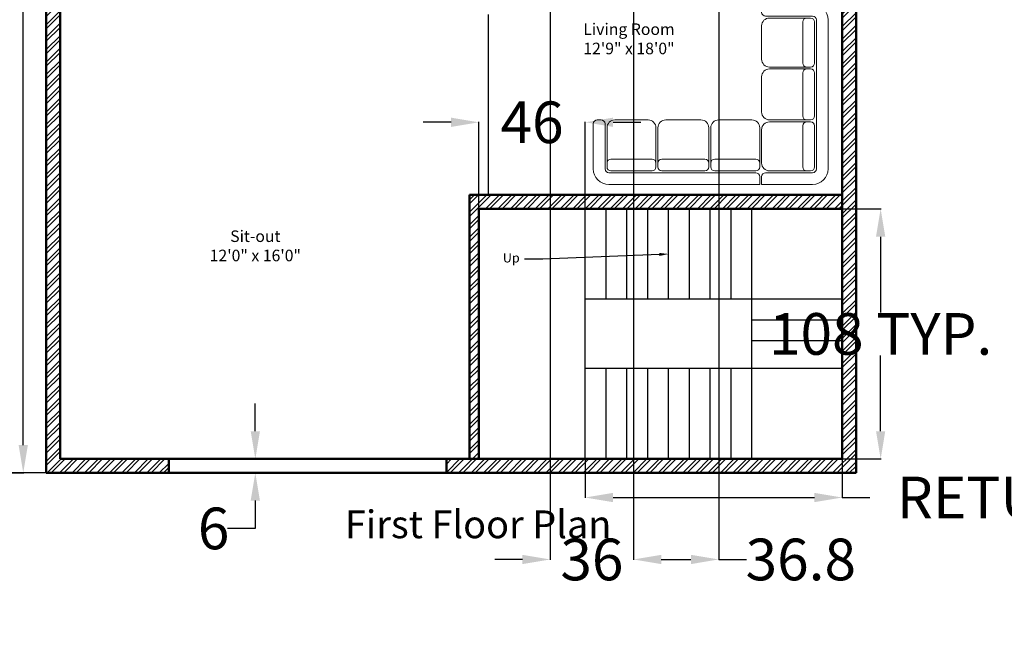
# Model space of a CAD drawing. Units: inches. Extents: x 73 to 1216, y -495 to 328.
# Tile 4 of 9: x 569 to 994, y -495 to -232. Entities that reach past the tile are written whole.
import ezdxf
from ezdxf import colors
from ezdxf.entities.mleader import LeaderData, LeaderLine
from ezdxf.math import Vec2, Vec3

# ---------------------------------------------------------------- set-up
doc = ezdxf.new("R2010")
doc.units = ezdxf.units.IN
for name, color, linetype, lineweight in [('A-ANNO-DIMS', 2, 'Continuous', 18), ('A-ANNO-TITL', 7, 'Continuous', 35), ('A-AREA-IDEN', 7, 'Continuous', 18), ('A-FLOR-EDGE', 7, 'Continuous', 25), ('A-WALL-PATT', 8, 'Continuous', 13), ('Furniture', 2, 'Continuous', 18), ('Outer Walls', 1, 'Continuous', 50), ('Stairs', 8, 'Continuous', 25), ('Text-T18', 7, 'Continuous', 18)]:
    doc.layers.add(name, color=color, linetype=linetype, lineweight=lineweight)
doc.styles.get("Standard").update_dxf_attribs({"font": 'arial.ttf'})
doc.dimstyles.get("Standard").update_dxf_attribs({"dimtxt": 18, "dimasz": 12, "dimexe": 0.18, "dimexo": 0.0625, "dimgap": 0.09, "dimtad": 0, "dimtih": 1, "dimtoh": 1, "dimdec": 0, "dimzin": 0, "dimdsep": 46, "dimlunit": 3, "dimtxsty": 'Standard', "dimcen": 0.09, "dimadec": 0, "dimazin": 0, "dimtfac": 1, "dimtdec": 0, "dimtofl": 0, "dimtmove": 0, "dimatfit": 3, "dimfxl": 1, "dimtolj": 1, "dimtzin": 0, "dimarcsym": 0})
pattern_1 = [(45, (-647.324, -1257.0093), (-2.694077, 2.694077), []), (45, (-645.528, -1257.0093), (-2.694077, 2.694077), [])]

# ---------------------------------------------------------------- blocks, each defined once
blk = doc.blocks.new('A$C2AFA021D')
for p, q in [((0.8, 2.3), (0.2, 2.3)), ((0.2, 2.15), (0.8, 2.15)), ((0.85, 2.2), (0.85, 2.25)), ((0, 2.1), (0, 0.2)), ((0.15, 0.2), (0.15, 2.1)), ((0.175, 1.55), (0.175, 2.075)), ((0.225, 2.125), (0.275, 2.125)), ((0.75, 2.125), (0.275, 2.125)), ((0.325, 2.075), (0.325, 1.55)), ((0.85, 1.6), (0.85, 2.025)), ((0.175, 0.875), (0.175, 1.425)), ((0.275, 1.5), (0.225, 1.5)), ((0.225, 1.475), (0.275, 1.475)), ((0.275, 1.5), (0.75, 1.5)), ((0.75, 1.475), (0.275, 1.475)), ((0.325, 1.425), (0.325, 0.875)), ((0.85, 0.925), (0.85, 1.375)), ((0.275, 0.825), (0.225, 0.825)), ((0.225, 0.8), (0.275, 0.8)), ((0.275, 0.825), (0.75, 0.825)), ((0.75, 0.8), (0.275, 0.8)), ((0.975, 0.825), (1.4, 0.825)), ((1.625, 0.825), (2.075, 0.825)), ((2.3, 0.825), (2.725, 0.825)), ((2.85, 0.2), (2.85, 0.775)), ((2.9, 0.825), (2.95, 0.825)), ((3, 0.775), (3, 0.2)), ((0.175, 0.225), (0.175, 0.75)), ((0.325, 0.75), (0.325, 0.225)), ((0.85, 0.275), (0.85, 0.7)), ((0.875, 0.275), (0.875, 0.725)), ((1.5, 0.725), (1.5, 0.275)), ((1.525, 0.275), (1.525, 0.725)), ((2.175, 0.725), (2.175, 0.275)), ((2.2, 0.275), (2.2, 0.725)), ((2.825, 0.725), (2.825, 0.275)), ((0.875, 0.275), (0.875, 0.225)), ((1.45, 0.325), (0.925, 0.325)), ((1.5, 0.225), (1.5, 0.275)), ((1.525, 0.275), (1.525, 0.225)), ((2.125, 0.325), (1.575, 0.325)), ((2.175, 0.225), (2.175, 0.275)), ((2.2, 0.275), (2.2, 0.225)), ((2.775, 0.325), (2.25, 0.325)), ((2.825, 0.225), (2.825, 0.275)), ((0.8, 0.15), (0.2, 0.15)), ((0.275, 0.175), (0.225, 0.175)), ((0.275, 0.175), (0.75, 0.175)), ((0.925, 0.175), (1.45, 0.175)), ((0.925, 0.15), (2.8, 0.15)), ((1.575, 0.175), (2.125, 0.175)), ((2.25, 0.175), (2.775, 0.175)), ((0.85, 0), (0.85, 0.1)), ((0.875, 0.1), (0.875, 0)), ((0.2, 0), (0.85, 0)), ((2.8, 0), (0.875, 0))]:
    blk.add_line(p, q)
for centre, radius, start, end in [((0.2, 2.1), 0.2, 90, 180), ((0.8, 2.25), 0.05, 0, 90), ((0.2, 2.1), 0.05, 90, 180), ((0.8, 2.2), 0.05, 270, 0), ((0.225, 2.075), 0.05, 90, 180), ((0.275, 2.075), 0.05, 0, 90), ((0.75, 2.025), 0.1, 0, 90), ((0.225, 1.55), 0.05, 180, 270), ((0.275, 1.55), 0.05, 270, 0), ((0.75, 1.6), 0.1, 270, 0), ((0.225, 1.425), 0.05, 90, 180), ((0.275, 1.425), 0.05, 0, 90), ((0.75, 1.375), 0.1, 360, 90), ((0.75, 0.925), 0.1, 270, 0), ((0.225, 0.875), 0.05, 180, 270), ((0.225, 0.75), 0.05, 90, 180), ((0.275, 0.875), 0.05, 270, 0), ((0.275, 0.75), 0.05, 0, 90), ((0.75, 0.7), 0.1, 0, 90), ((0.975, 0.725), 0.1, 90, 180), ((1.4, 0.725), 0.1, 0, 90), ((1.625, 0.725), 0.1, 90, 180), ((2.075, 0.725), 0.1, 0, 90), ((2.3, 0.725), 0.1, 90, 180), ((2.725, 0.725), 0.1, 0, 90), ((2.9, 0.775), 0.05, 90, 180), ((2.95, 0.775), 0.05, 0, 90), ((0.75, 0.275), 0.1, 270, 0), ((0.925, 0.275), 0.05, 90, 180), ((1.45, 0.275), 0.05, 360, 90), ((1.575, 0.275), 0.05, 90, 180), ((2.125, 0.275), 0.05, 360, 90), ((2.25, 0.275), 0.05, 90, 180), ((2.775, 0.275), 0.05, 360, 90), ((0.2, 0.2), 0.2, 180, 270), ((0.2, 0.2), 0.05, 180, 270), ((0.225, 0.225), 0.05, 180, 270), ((0.275, 0.225), 0.05, 270, 0), ((0.8, 0.1), 0.05, 0, 90), ((0.925, 0.225), 0.05, 180, 270), ((0.925, 0.1), 0.05, 90, 180), ((1.45, 0.225), 0.05, 270, 0), ((1.575, 0.225), 0.05, 180, 270), ((2.125, 0.225), 0.05, 270, 0), ((2.25, 0.225), 0.05, 180, 270), ((2.775, 0.225), 0.05, 270, 0), ((2.8, 0.2), 0.2, 270, 0), ((2.8, 0.2), 0.05, 270, 0)]:
    blk.add_arc(centre, radius, start, end)
blk = doc.blocks.new('STAIR-RETURN')
for p, q in [((0, 69), (0, 108)), ((9, 69), (9, 108)), ((18, 69), (18, 108)), ((27, 69), (27, 108)), ((36, 69), (36, 108)), ((45, 69), (45, 108)), ((54, 69), (54, 108)), ((63, 69), (63, 108)), ((72, 0), (72, 108)), ((111, 69), (0, 69)), ((0, 0), (0, 69)), ((111, 60), (72, 60)), ((111, 51), (72, 51)), ((111, 39), (0, 39)), ((9, 0), (9, 39)), ((18, 0), (18, 39)), ((27, 0), (27, 39)), ((36, 0), (36, 39)), ((45, 0), (45, 39)), ((54, 0), (54, 39)), ((63, 0), (63, 39))]:
    blk.add_line(p, q)
blk = doc.blocks.new('*D46')
at = {"layer": 'A-ANNO-DIMS', "color": 0, "lineweight": -2, "transparency": 16777216}
for p, q in [((813.16, -421.89), (813.16, -438.65)), ((924.16, -421.89), (924.16, -438.65)), ((825.16, -438.47), (912.16, -438.47)), ((924.16, -438.47), (936.16, -438.47))]:
    blk.add_line(p, q, dxfattribs=at)
at = {"layer": 'A-ANNO-DIMS', "color": 0, "transparency": 16777216}
for points in [[(825.16, -436.47), (825.16, -440.47), (813.16, -438.47)], [(912.16, -436.47), (912.16, -440.47), (924.16, -438.47)]]:
    blk.add_solid(points, dxfattribs=at)
at = {"layer": 'Defpoints', "color": 0, "transparency": 16777216}
for p in [(813.16, -421.82), (924.16, -421.82), (924.16, -438.47)]:
    blk.add_point(p, dxfattribs=at)
at = {"layer": 'A-ANNO-DIMS', "color": 0, "transparency": 16777216, "insert": (1082.99, -438.47), "char_height": 18, "attachment_point": 5}
blk.add_mtext('\\A1;RETURN STAIR 111 TYP.', dxfattribs=at)
blk = doc.blocks.new('*D47')
at = {"layer": 'A-ANNO-DIMS', "color": 0, "lineweight": -2, "transparency": 16777216}
for p, q in [((924.23, -313.82), (940.99, -313.82)), ((940.81, -325.82), (940.81, -358.54)), ((940.81, -409.82), (940.81, -377.1)), ((924.23, -421.82), (940.99, -421.82))]:
    blk.add_line(p, q, dxfattribs=at)
at = {"layer": 'A-ANNO-DIMS', "color": 0, "transparency": 16777216}
for points in [[(938.81, -325.82), (942.81, -325.82), (940.81, -313.82)], [(938.81, -409.82), (942.81, -409.82), (940.81, -421.82)]]:
    blk.add_solid(points, dxfattribs=at)
at = {"layer": 'Defpoints', "color": 0, "transparency": 16777216}
for p in [(924.16, -313.82), (940.81, -313.82), (924.16, -421.82)]:
    blk.add_point(p, dxfattribs=at)
at = {"layer": 'A-ANNO-DIMS', "color": 0, "transparency": 16777216, "insert": (940.81, -367.82), "char_height": 18, "attachment_point": 5}
blk.add_mtext('\\A1;108 TYP.', dxfattribs=at)
blk = doc.blocks.new('*D51')
at = {"layer": 'A-ANNO-DIMS', "color": 0, "lineweight": -2, "transparency": 16777216}
for p, q in [((532.94, 279.18), (570.45, 279.18)), ((570.27, 267.18), (570.27, -65.04)), ((570.27, -415.82), (570.27, -83.6)), ((532.94, -427.82), (570.45, -427.82))]:
    blk.add_line(p, q, dxfattribs=at)
at = {"layer": 'A-ANNO-DIMS', "color": 0, "transparency": 16777216}
for points in [[(568.27, 267.18), (572.27, 267.18), (570.27, 279.18)], [(568.27, -415.82), (572.27, -415.82), (570.27, -427.82)]]:
    blk.add_solid(points, dxfattribs=at)
at = {"layer": 'Defpoints', "color": 0, "transparency": 16777216}
for p in [(532.87, 279.18), (570.27, 279.18), (532.87, -427.82)]:
    blk.add_point(p, dxfattribs=at)
at = {"layer": 'A-ANNO-DIMS', "color": 0, "transparency": 16777216, "insert": (570.27, -74.32), "char_height": 18, "attachment_point": 5}
blk.add_mtext('\\A1;707', dxfattribs=at)
blk = doc.blocks.new('*D53')
at = {"layer": 'A-ANNO-DIMS', "color": 0, "lineweight": -2, "transparency": 16777216}
for p, q in [((580.1, 279.18), (542.58, 279.18)), ((542.76, 267.18), (542.76, -65.04)), ((542.76, -415.82), (542.76, -83.6)), ((580.1, -427.82), (542.58, -427.82))]:
    blk.add_line(p, q, dxfattribs=at)
at = {"layer": 'A-ANNO-DIMS', "color": 0, "transparency": 16777216}
for points in [[(540.76, 267.18), (544.76, 267.18), (542.76, 279.18)], [(540.76, -415.82), (544.76, -415.82), (542.76, -427.82)]]:
    blk.add_solid(points, dxfattribs=at)
at = {"layer": 'Defpoints', "color": 0, "transparency": 16777216}
for p in [(542.76, 279.18), (580.16, 279.18), (580.16, -427.82)]:
    blk.add_point(p, dxfattribs=at)
at = {"layer": 'A-ANNO-DIMS', "color": 0, "transparency": 16777216, "insert": (542.76, -74.32), "char_height": 18, "attachment_point": 5}
blk.add_mtext('\\A1;707', dxfattribs=at)
blk = doc.blocks.new('*D66')
at = {"layer": 'A-ANNO-DIMS', "color": 0, "lineweight": -2, "transparency": 16777216}
for p, q in [((755.164694, -276.423699), (743.164694, -276.423699)), ((767.164694, -313.761199), (767.164694, -276.243699)), ((813.164694, -313.761199), (813.164694, -276.243699)), ((825.164694, -276.423699), (837.164694, -276.423699))]:
    blk.add_line(p, q, dxfattribs=at)
at = {"layer": 'A-ANNO-DIMS', "color": 0, "transparency": 16777216}
for points in [[(755.164694, -274.423699), (755.164694, -278.423699), (767.164694, -276.423699)], [(825.164694, -274.423699), (825.164694, -278.423699), (813.164694, -276.423699)]]:
    blk.add_solid(points, dxfattribs=at)
at = {"layer": 'Defpoints', "color": 0, "transparency": 16777216}
for p in [(813.164694, -276.423699), (767.164694, -313.823699), (813.164694, -313.823699)]:
    blk.add_point(p, dxfattribs=at)
at = {"layer": 'A-ANNO-DIMS', "color": 0, "transparency": 16777216, "insert": (790.164694, -276.423699), "char_height": 18, "attachment_point": 5}
blk.add_mtext('\\A1;46', dxfattribs=at)
blk = doc.blocks.new('*D67')
at = {"layer": 'A-ANNO-DIMS', "color": 0, "lineweight": -2, "transparency": 16777216}
for p, q in [((798.02113, 227.113801), (798.02113, -465.403699)), ((834.02113, 227.113801), (834.02113, -465.403699)), ((786.02113, -465.223699), (774.02113, -465.223699)), ((846.02113, -465.223699), (858.02113, -465.223699))]:
    blk.add_line(p, q, dxfattribs=at)
at = {"layer": 'A-ANNO-DIMS', "color": 0, "transparency": 16777216}
for points in [[(786.02113, -463.223699), (786.02113, -467.223699), (798.02113, -465.223699)], [(846.02113, -463.223699), (846.02113, -467.223699), (834.02113, -465.223699)]]:
    blk.add_solid(points, dxfattribs=at)
at = {"layer": 'Defpoints', "color": 0, "transparency": 16777216}
for p in [(798.02113, 227.176301), (834.02113, 227.176301), (834.02113, -465.223699)]:
    blk.add_point(p, dxfattribs=at)
at = {"layer": 'A-ANNO-DIMS', "color": 0, "transparency": 16777216, "insert": (816.02113, -465.223699), "char_height": 18, "attachment_point": 5}
blk.add_mtext('\\A1;36', dxfattribs=at)
blk = doc.blocks.new('*D68')
at = {"layer": 'A-ANNO-DIMS', "color": 0, "lineweight": -2, "transparency": 16777216}
for p, q in [((834.02, 227.11), (834.02, -465.4)), ((870.82, 227.11), (870.82, -465.4)), ((846.02, -465.22), (858.82, -465.22)), ((870.82, -465.22), (882.82, -465.22))]:
    blk.add_line(p, q, dxfattribs=at)
at = {"layer": 'A-ANNO-DIMS', "color": 0, "transparency": 16777216}
for points in [[(846.02, -463.22), (846.02, -467.22), (834.02, -465.22)], [(858.82, -463.22), (858.82, -467.22), (870.82, -465.22)]]:
    blk.add_solid(points, dxfattribs=at)
at = {"layer": 'Defpoints', "color": 0, "transparency": 16777216}
for p in [(834.02, 227.18), (870.82, 227.18), (870.82, -465.22)]:
    blk.add_point(p, dxfattribs=at)
at = {"layer": 'A-ANNO-DIMS', "color": 0, "transparency": 16777216, "insert": (906.3, -465.22), "char_height": 18, "attachment_point": 5}
blk.add_mtext('\\A1;36.8', dxfattribs=at)
blk = doc.blocks.new('*D70')
at = {"layer": 'A-ANNO-DIMS', "color": 0, "lineweight": -2, "transparency": 16777216}
for p, q in [((670.56, -409.82), (670.56, -397.82)), ((633.23, -421.82), (670.74, -421.82)), ((633.23, -427.82), (670.74, -427.82)), ((670.56, -439.82), (670.56, -451.82)), ((670.56, -451.82), (658.56, -451.82))]:
    blk.add_line(p, q, dxfattribs=at)
at = {"layer": 'A-ANNO-DIMS', "color": 0, "transparency": 16777216}
for points in [[(668.56, -409.82), (672.56, -409.82), (670.56, -421.82)], [(668.56, -439.82), (672.56, -439.82), (670.56, -427.82)]]:
    blk.add_solid(points, dxfattribs=at)
at = {"layer": 'Defpoints', "color": 0, "transparency": 16777216}
for p in [(633.16, -421.82), (633.16, -427.82), (670.56, -427.82)]:
    blk.add_point(p, dxfattribs=at)
at = {"layer": 'A-ANNO-DIMS', "color": 0, "transparency": 16777216, "insert": (652.53, -451.82), "char_height": 18, "attachment_point": 5}
blk.add_mtext('\\A1;6', dxfattribs=at)

msp = doc.modelspace()

# ---------------------------------------------------------------- hatches: boundary and pattern name
at = {"layer": 'A-WALL-PATT'}
h = msp.add_hatch(dxfattribs=at)
h.set_pattern_fill('ANSI32', color=256, scale=0.4)
h.set_pattern_definition(pattern_1)
h.paths.add_polyline_path([(586.1647, 273.1763), (924.1647, 273.1763), (924.1647, -421.8237), (753.1647, -421.8237), (753.1647, -427.8237), (930.1647, -427.8237), (930.1647, 279.1763), (580.1647, 279.1763), (580.1647, -427.8237), (633.1647, -427.8237), (633.1647, -421.8237), (586.1647, -421.8237)])
h = msp.add_hatch(dxfattribs=at)
h.set_pattern_fill('ANSI32', color=256, scale=0.4)
h.set_pattern_definition(pattern_1)
h.paths.add_polyline_path([(685.1647, 201.1763), (679.1647, 201.1763), (679.1647, 206.1763), (675.1647, 206.1763), (675.1647, 201.1763), (586.1647, 201.1763), (586.1647, 197.1763), (685.1647, 197.1763)])
h.paths.add_polyline_path([(679.1647, 273.1763), (675.1647, 273.1763), (675.1647, 236.1763), (679.1647, 236.1763)])
h.paths.add_polyline_path([(775.1647, 201.1763), (772.1647, 201.1763), (772.1647, 273.1763), (768.1647, 273.1763), (768.1647, 249.1763), (768.1647, 201.1763), (721.1647, 201.1763), (721.1647, 197.1763), (771.1647, 197.1763), (771.1647, 58.1763), (775.1647, 58.1763)])
h.paths.add_polyline_path([(798.0211, 233.1763), (772.1647, 233.1763), (772.1647, 227.1763), (798.0211, 227.1763)])
h.paths.add_polyline_path([(870.8232, 233.1763), (834.0211, 233.1763), (834.0211, 227.1763), (870.8232, 227.1763)])
h.paths.add_polyline_path([(924.1647, 233.1763), (906.8232, 233.1763), (906.8232, 227.1763), (924.1647, 227.1763)])
h.paths.add_polyline_path([(924.1647, 83.1763), (775.1647, 83.1763), (775.1647, 79.1763), (924.1647, 79.1763)])
h.paths.add_polyline_path([(775.1647, 22.1763), (771.1647, 22.1763), (771.1647, 16.1763), (628.1647, 16.1763), (628.1647, 12.1763), (775.1647, 12.1763)])
h.paths.add_polyline_path([(692.1647, 12.1763), (688.1647, 12.1763), (688.1647, -52.8237), (692.1647, -52.8237)])
h.paths.add_polyline_path([(924.1647, 39.1763), (824.1647, 39.1763), (824.1647, 35.1763), (924.1647, 35.1763)])
h.paths.add_polyline_path([(874.6647, -29.8237), (864.1647, -29.8237), (824.1647, -29.8237), (824.1647, -87.8237), (817.1647, -87.8237), (817.1647, -91.8237), (844.6647, -91.8237), (844.6647, -87.8237), (828.1647, -87.8237), (828.1647, -33.8237), (874.6647, -33.8237)])
h.paths.add_polyline_path([(924.1647, -29.8237), (910.6647, -29.8237), (910.6647, -33.8237), (924.1647, -33.8237)])
h.paths.add_polyline_path([(924.1647, -87.8237), (904.6647, -87.8237), (904.6647, -91.8237), (924.1647, -91.8237)])
h.paths.add_polyline_path([(777.1647, -88.8237), (761.1647, -88.8237), (761.1647, -92.8237), (767.1647, -92.8237), (767.1647, -224.8237), (771.1647, -224.8237), (771.1647, -92.8237), (777.1647, -92.8237)])
h.paths.add_polyline_path([(725.1647, -88.8237), (628.1647, -88.8237), (628.1647, -92.8237), (725.1647, -92.8237)])
h.paths.add_polyline_path([(692.1647, -82.8237), (688.1647, -82.8237), (688.1647, -88.8237), (692.1647, -88.8237)])
h.paths.add_polyline_path([(767.1647, -313.8237), (924.1647, -313.8237), (924.1647, -307.8237), (763.1647, -307.8237), (763.1647, -421.8237), (767.1647, -421.8237)])

# ---------------------------------------------------------------- linework, layer by layer
at = {"layer": 'A-FLOR-EDGE'}
msp.add_line((771.1647, -229.8237), (771.1647, -307.8237), dxfattribs=at)
at = {"layer": 'Outer Walls'}
for p, q in [((580.1647, -427.8237), (580.1647, 279.1763)), ((930.1647, -427.8237), (930.1647, 279.1763)), ((586.1647, -421.8237), (586.1647, 273.1763)), ((924.1647, -421.8237), (924.1647, 273.1763)), ((924.1647, -307.8237), (763.1647, -307.8237)), ((763.1647, -421.8237), (763.1647, -307.8237)), ((924.1647, -313.8237), (767.1647, -313.8237)), ((767.1647, -421.8237), (767.1647, -313.8237)), ((924.1647, -421.8237), (586.1647, -421.8237)), ((633.1647, -427.8237), (633.1647, -421.8237)), ((753.1647, -427.8237), (753.1647, -421.8237)), ((930.1647, -427.8237), (580.1647, -427.8237))]:
    msp.add_line(p, q, dxfattribs=at)

# ---------------------------------------------------------------- block references
at = {"layer": 'Furniture', "xscale": -33.84012530478223, "yscale": 33.84012530478223, "zscale": 33.84012530478223}
msp.add_blockref('A$C2AFA021D', (918.1526, -303.3147), dxfattribs=at)
at = {"layer": 'Stairs'}
msp.add_blockref('STAIR-RETURN', (813.1647, -421.8237), dxfattribs=at)

# ---------------------------------------------------------------- texts
at = {"layer": 'A-ANNO-TITL', "insert": (845.3747, -444.0461), "char_height": 12, "attachment_point": 3}
msp.add_mtext_dynamic_manual_height_columns('\\pxqc;{\\fTimes New Roman|b0|i0|c0|p18;First Floor Plan}', width=157.002992, gutter_width=12.5, heights=[0], dxfattribs=at)
at = {"layer": 'A-AREA-IDEN', "char_height": 5, "attachment_point": 3}
for s, insert in [('\\pxqc;{\\fTimes New Roman|b0|i0|c0|p18;Living Room\\P12\'9" x 18\'0"}', (856.5878, -233.7148)), ('\\pxqc;{\\fTimes New Roman|b0|i0|c0|p18;Sit-out\\P12\'0" x 16\'0"}', (695.1186, -323.1138))]:
    msp.add_mtext_dynamic_manual_height_columns(s, width=49.101878, gutter_width=12.5, heights=[0], dxfattribs=dict(at, insert=insert))

# ---------------------------------------------------------------- dimensions: what is measured, and where the dimension line sits
at = {"layer": 'A-ANNO-DIMS'}
for base, p1, p2, angle, picture, middle in [((542.7647, 279.1763), (580.1647, -427.8237), (580.1647, 279.1763), 90, '*D53', (542.7647, -74.3237)), ((570.2746, 279.1763), (532.8746, -427.8237), (532.8746, 279.1763), 90, '*D51', (570.2746, -74.3237)), ((670.5647, -427.8237), (633.1647, -421.8237), (633.1647, -427.8237), 270, '*D70', (652.532, -451.8237))]:
    dim = msp.add_linear_dim(base=base, p1=p1, p2=p2, angle=angle, dimstyle='Standard', override={"dimdec": 0, "dimlfac": 1, "dimrnd": 0, "dimzin": 0, "dimdsep": 46, "dimlunit": 2}, dxfattribs=at)
    dim.commit()
    dim.dimension.update_dxf_attribs({"geometry": picture, "text_midpoint": middle})
for base, p1, p2, override, picture, middle in [((834.0211, -465.2237), (798.0211, 227.1763), (834.0211, 227.1763), {"dimdec": 0, "dimlfac": 1, "dimrnd": 0, "dimzin": 0, "dimdsep": 46, "dimlunit": 2}, '*D67', (816.0211, -465.2237)), ((870.8232, -465.2237), (834.0211, 227.1763), (870.8232, 227.1763), {"dimdec": 1, "dimlfac": 1, "dimrnd": 0, "dimzin": 0, "dimdsep": 46, "dimlunit": 2}, '*D68', (906.3033, -465.2237)), ((813.1647, -276.4237), (767.1647, -313.8237), (813.1647, -313.8237), {"dimdec": 0, "dimlfac": 1, "dimrnd": 0, "dimzin": 0, "dimdsep": 46, "dimlunit": 2}, '*D66', (790.1647, -276.4237))]:
    dim = msp.add_linear_dim(base=base, p1=p1, p2=p2, dimstyle='Standard', override=override, dxfattribs=at)
    dim.commit()
    dim.dimension.update_dxf_attribs({"geometry": picture, "text_midpoint": middle})
dim = msp.add_linear_dim(base=(940.8147, -313.8237), p1=(924.1647, -421.8237), p2=(924.1647, -313.8237), angle=90, text='<> TYP.', dimstyle='Standard', override={"dimdec": 0, "dimlfac": 1, "dimrnd": 0, "dimzin": 0, "dimdsep": 46, "dimlunit": 2}, dxfattribs=at)
dim.commit()
dim.dimension.update_dxf_attribs({"geometry": '*D47', "text_midpoint": (940.8147, -367.8237)})
dim = msp.add_linear_dim(base=(924.1647, -438.4737), p1=(813.1647, -421.8237), p2=(924.1647, -421.8237), text='RETURN STAIR <> TYP.', dimstyle='Standard', override={"dimdec": 0, "dimlfac": 1, "dimrnd": 0, "dimzin": 0, "dimdsep": 46, "dimlunit": 2}, dxfattribs=at)
dim.commit()
dim.dimension.update_dxf_attribs({"geometry": '*D46', "text_midpoint": (1082.9866, -438.4737)})

# ---------------------------------------------------------------- leaders
at = {"layer": 'Text-T18'}
ml = msp.add_multileader_mtext('Standard', dxfattribs=at)
ml.set_content('{\\fTimes New Roman|b0|i0|c0|p18;Up}', color=256)
ml.set_leader_properties()
ml.build(insert=Vec2(0, 0))
ctx = ml.context
ctx.base_point, ctx.plane_origin = Vec3(775.8383, -335.5898), Vec3(849.1647, -333.3237)
ctx.text_align_type = 2
notes = []
notes.append((ctx, [(0, (1, 1, 0), (794.8232, -335.5898), (-1, 0), 8, [(0, [(849.1647, -333.3237)], 0, [])])]))
ctx.mtext.insert, ctx.mtext.alignment, ctx.mtext.flow_direction = Vec3(784.8232, -332.9582), 3, 5
for ctx, leaders in notes:
    for number, flags, end, landing, length, lines in leaders:
        leader = LeaderData()
        leader.index, (leader.has_last_leader_line, leader.has_dogleg_vector, leader.attachment_direction) = number, flags
        leader.last_leader_point, leader.dogleg_vector, leader.dogleg_length = Vec3(end), Vec3(landing), length
        for number, points, colour, breaks in lines:
            line = LeaderLine()
            line.index, line.vertices, line.color, line.breaks = number, Vec3.list(points), colors.encode_raw_color(colour), breaks
            leader.lines.append(line)
        ctx.leaders.append(leader)

doc.saveas('drawing.dxf')
